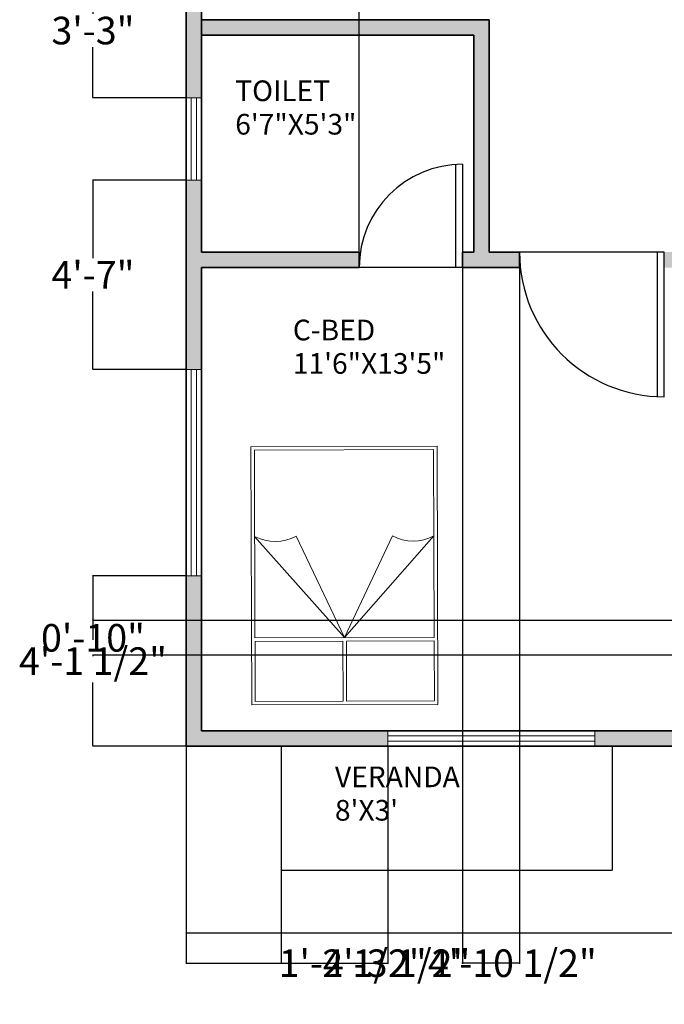
# Model space of a CAD drawing. Units: inches. Extents: x -27 to 662, y -19 to 539.
# Tile 1 of 4: x -27 to 160, y -19 to 267. Entities that reach past the tile are written whole.
import ezdxf

# ---------------------------------------------------------------- set-up
doc = ezdxf.new("R2010")
doc.units = ezdxf.units.IN
doc.header["$MEASUREMENT"] = 0
for name, color, linetype, lineweight in [('A-ANNO-DIMS', 2, 'Continuous', 18), ('A-AREA-IDEN', 230, 'Continuous', 18), ('A-DOOR', 6, 'Continuous', 25), ('A-FLOR', 4, 'Continuous', 25), ('A-FURN', 240, 'Continuous', 18), ('A-GLAZ', 240, 'Continuous', 18), ('A-WALL', 4, 'Continuous', 35)]:
    doc.layers.add(name, color=color, linetype=linetype, lineweight=lineweight)
doc.layers.add('A-WALL-PATT', color=2, linetype='Continuous', lineweight=13, true_color=0xf1eb1f)
doc.styles.get("Standard").update_dxf_attribs({"font": 'italic8.shx'})
doc.dimstyles.get("Standard").update_dxf_attribs({"dimtxt": 8, "dimasz": 0.18, "dimexe": 0.18, "dimexo": 0.0625, "dimgap": 0.09, "dimtad": 0, "dimtih": 1, "dimtoh": 1, "dimzin": 0, "dimdsep": 46, "dimlunit": 3, "dimtxsty": 'Standard', "dimcen": 0.09, "dimclrt": 4, "dimadec": 0, "dimazin": 0, "dimtfac": 1, "dimtofl": 0, "dimtmove": 0, "dimatfit": 3, "dimfxl": 1, "dimtolj": 1, "dimtzin": 0, "dimarcsym": 0})

# ---------------------------------------------------------------- blocks, each defined once
blk = doc.blocks.new('*D1')
at = {"layer": 'A-ANNO-DIMS', "color": 0, "lineweight": -2, "transparency": 16777216}
for p, q in [((21.29, 55.86), (21.29, 1.58)), ((417.29, 55.86), (417.29, 1.58)), ((21.47, 1.76), (209.67, 1.76)), ((417.11, 1.76), (228.9, 1.76))]:
    blk.add_line(p, q, dxfattribs=at)
at = {"layer": 'A-ANNO-DIMS', "color": 0, "transparency": 16777216}
for points in [[(21.47, 1.79), (21.47, 1.73), (21.29, 1.76)], [(417.11, 1.79), (417.11, 1.73), (417.29, 1.76)]]:
    blk.add_solid(points, dxfattribs=at)
at = {"layer": 'Defpoints', "color": 0, "transparency": 16777216}
for p in [(21.29, 55.92), (417.29, 55.92), (417.29, 1.76)]:
    blk.add_point(p, dxfattribs=at)
at = {"layer": 'A-ANNO-DIMS', "color": 0, "transparency": 16777216, "insert": (219.29, 1.76), "char_height": 8, "attachment_point": 5}
blk.add_mtext("\\A1;33'", dxfattribs=at)
blk = doc.blocks.new('BED-DOUBLE-54x75')
for p, q in [((26.5, 56.54), (26.5, 74)), ((27.5, 56.54), (27.5, 74)), ((1, 56.54), (26.5, 56.54)), ((1, 55.54), (53, 55.54)), ((27, 55.54), (1, 26.04)), ((13, 26.04), (27, 55.54)), ((27, 55.54), (53, 26.04)), ((41, 26.04), (27, 55.54)), ((27.5, 56.54), (53, 56.54))]:
    blk.add_line(p, q)
blk.add_lwpolyline([(0, 75), (54, 75), (54, 0), (0, 0)], close=True)
for points in [[(1, 56.54), (1, 74), (26.5, 74)], [(27.5, 74), (53, 74), (53, 56.54)], [(53, 55.54), (53, 1), (1, 1), (1, 55.54)]]:
    blk.add_lwpolyline(points)
for centre in [(7, 14.92), (47, 14.92)]:
    blk.add_arc(centre, 12.64, 61.656, 118.344)
blk = doc.blocks.new('DOOR-SWING-30IN')
for p, q in [((28, 29.93), (28, 0)), ((30, 30), (30, 0)), ((30, 0), (0, 0))]:
    blk.add_line(p, q)
blk.add_arc((30, 0), 30, 90, 180)
blk = doc.blocks.new('DOOR-SWING-42IN')
for p, q in [((0, 42), (0, 0)), ((2, 41.95), (2, 0)), ((0, 0), (42, 0))]:
    blk.add_line(p, q)
blk.add_arc((0, 0), 42, 0, 90)
blk = doc.blocks.new('WIN-60IN')
for p, q in [((0, 4.5), (0, 0)), ((60, 4.5), (0, 4.5)), ((0, 3), (60, 3)), ((60, 0), (60, 4.5)), ((0, 1.5), (60, 1.5)), ((0, 0), (60, 0))]:
    blk.add_line(p, q)
blk = doc.blocks.new('WIN-60IN-B')
for p, q in [((0, 0), (0, 60)), ((0, 60), (4.5, 60)), ((1.5, 0), (1.5, 60)), ((3, 0), (3, 60)), ((4.5, 60), (4.5, 0)), ((4.5, 0), (0, 0)), ((4.5, 0), (2.25, 0))]:
    blk.add_line(p, q)
blk = doc.blocks.new('WIN-24IN-B')
for p, q in [((0, 24), (4.5, 24)), ((0, 0), (0, 24)), ((0, 24), (2.25, 24)), ((1.5, 24), (1.5, 0)), ((3, 24), (3, 0)), ((4.5, 24), (4.5, 0)), ((4.5, 0), (0, 0))]:
    blk.add_line(p, q)
blk = doc.blocks.new('*D25')
at = {"layer": 'A-ANNO-DIMS', "color": 0, "lineweight": -2, "transparency": 16777216}
for p, q in [((21.29, 283.19), (21.29, 277.67)), ((25.79, 283.19), (25.79, 277.67)), ((21.47, 277.85), (25.61, 277.85)), ((25.79, 277.85), (25.97, 277.85))]:
    blk.add_line(p, q, dxfattribs=at)
at = {"layer": 'A-ANNO-DIMS', "color": 0, "transparency": 16777216}
for points in [[(21.47, 277.88), (21.47, 277.82), (21.29, 277.85)], [(25.61, 277.88), (25.61, 277.82), (25.79, 277.85)]]:
    blk.add_solid(points, dxfattribs=at)
at = {"layer": 'Defpoints', "color": 0, "transparency": 16777216}
for p in [(21.29, 283.25), (25.79, 283.25), (25.79, 277.85)]:
    blk.add_point(p, dxfattribs=at)
at = {"layer": 'A-ANNO-DIMS', "color": 4, "transparency": 16777216, "insert": (77.49, 277.85), "char_height": 8, "attachment_point": 5}
blk.add_mtext('\\A1;0\'-4 1/2" TYP.', dxfattribs=at)
blk = doc.blocks.new('*D36')
at = {"layer": 'A-ANNO-DIMS', "color": 0, "lineweight": -2, "transparency": 16777216}
for p, q in [((168.225254, 92.419463), (-5.892246, 92.419463)), ((-5.712246, 92.599463), (-5.712246, 92.779463)), ((168.225254, 82.419463), (-5.892246, 82.419463)), ((-5.712246, 82.239463), (-5.712246, 82.059463))]:
    blk.add_line(p, q, dxfattribs=at)
at = {"layer": 'A-ANNO-DIMS', "color": 0, "transparency": 16777216}
for points in [[(-5.742246, 92.599463), (-5.682246, 92.599463), (-5.712246, 92.419463)], [(-5.742246, 82.239463), (-5.682246, 82.239463), (-5.712246, 82.419463)]]:
    blk.add_solid(points, dxfattribs=at)
at = {"layer": 'Defpoints', "color": 0, "transparency": 16777216}
for p in [(-5.712246, 92.419463), (168.287754, 92.419463), (168.287754, 82.419463)]:
    blk.add_point(p, dxfattribs=at)
at = {"layer": 'A-ANNO-DIMS', "color": 4, "transparency": 16777216, "insert": (-5.712246, 87.419463), "char_height": 8, "attachment_point": 5}
blk.add_mtext('\\A1;0\'-10"', dxfattribs=at)
blk = doc.blocks.new('*D45')
at = {"layer": 'A-ANNO-DIMS', "color": 0, "lineweight": -2, "transparency": 16777216}
for p, q in [((21.23, 105.38), (-5.89, 105.38)), ((-5.71, 105.2), (-5.71, 86.84)), ((-5.71, 56.1), (-5.71, 74.47)), ((21.23, 55.92), (-5.89, 55.92))]:
    blk.add_line(p, q, dxfattribs=at)
at = {"layer": 'A-ANNO-DIMS', "color": 0, "transparency": 16777216}
for points in [[(-5.74, 105.2), (-5.68, 105.2), (-5.71, 105.38)], [(-5.74, 56.1), (-5.68, 56.1), (-5.71, 55.92)]]:
    blk.add_solid(points, dxfattribs=at)
at = {"layer": 'Defpoints', "color": 0, "transparency": 16777216}
for p in [(-5.71, 105.38), (21.29, 105.38), (21.29, 55.92)]:
    blk.add_point(p, dxfattribs=at)
at = {"layer": 'A-ANNO-DIMS', "color": 4, "transparency": 16777216, "insert": (-5.71, 80.65), "char_height": 8, "attachment_point": 5}
blk.add_mtext('\\A1;4\'-1 1/2"', dxfattribs=at)
blk = doc.blocks.new('*D46')
at = {"layer": 'A-ANNO-DIMS', "color": 0, "lineweight": -2, "transparency": 16777216}
for p, q in [((21.23, 220.27), (-5.89, 220.27)), ((-5.71, 220.09), (-5.71, 197.68)), ((-5.71, 165.56), (-5.71, 187.98)), ((21.23, 165.38), (-5.89, 165.38))]:
    blk.add_line(p, q, dxfattribs=at)
at = {"layer": 'A-ANNO-DIMS', "color": 0, "transparency": 16777216}
for points in [[(-5.74, 220.09), (-5.68, 220.09), (-5.71, 220.27)], [(-5.74, 165.56), (-5.68, 165.56), (-5.71, 165.38)]]:
    blk.add_solid(points, dxfattribs=at)
at = {"layer": 'Defpoints', "color": 0, "transparency": 16777216}
for p in [(-5.71, 220.27), (21.29, 220.27), (21.29, 165.38)]:
    blk.add_point(p, dxfattribs=at)
at = {"layer": 'A-ANNO-DIMS', "color": 4, "transparency": 16777216, "insert": (-5.71, 192.83), "char_height": 8, "attachment_point": 5}
blk.add_mtext('\\A1;4\'-7"', dxfattribs=at)
blk = doc.blocks.new('*D47')
at = {"layer": 'A-ANNO-DIMS', "color": 0, "lineweight": -2, "transparency": 16777216}
for p, q in [((21.23, 283.25), (-5.89, 283.25)), ((-5.71, 283.07), (-5.71, 268.61)), ((-5.71, 244.45), (-5.71, 258.91)), ((21.23, 244.27), (-5.89, 244.27))]:
    blk.add_line(p, q, dxfattribs=at)
at = {"layer": 'A-ANNO-DIMS', "color": 0, "transparency": 16777216}
for points in [[(-5.74, 283.07), (-5.68, 283.07), (-5.71, 283.25)], [(-5.74, 244.45), (-5.68, 244.45), (-5.71, 244.27)]]:
    blk.add_solid(points, dxfattribs=at)
at = {"layer": 'Defpoints', "color": 0, "transparency": 16777216}
for p in [(-5.71, 283.25), (21.29, 283.25), (21.29, 244.27)]:
    blk.add_point(p, dxfattribs=at)
at = {"layer": 'A-ANNO-DIMS', "color": 4, "transparency": 16777216, "insert": (-5.71, 263.76), "char_height": 8, "attachment_point": 5}
blk.add_mtext('\\A1;3\'-3"', dxfattribs=at)
blk = doc.blocks.new('*D48')
at = {"layer": 'A-ANNO-DIMS', "color": 0, "lineweight": -2, "transparency": 16777216}
for p, q in [((21.29, 55.86), (21.29, -7.26)), ((79.87, 55.86), (79.87, -7.26)), ((21.47, -7.08), (79.69, -7.08)), ((79.87, -7.08), (80.05, -7.08))]:
    blk.add_line(p, q, dxfattribs=at)
at = {"layer": 'A-ANNO-DIMS', "color": 0, "transparency": 16777216}
for points in [[(21.47, -7.05), (21.47, -7.11), (21.29, -7.08)], [(79.69, -7.05), (79.69, -7.11), (79.87, -7.08)]]:
    blk.add_solid(points, dxfattribs=at)
at = {"layer": 'Defpoints', "color": 0, "transparency": 16777216}
for p in [(21.29, 55.92), (79.87, 55.92), (79.87, -7.08)]:
    blk.add_point(p, dxfattribs=at)
at = {"layer": 'A-ANNO-DIMS', "color": 4, "transparency": 16777216, "insert": (115.95, -7.08), "char_height": 8, "attachment_point": 5}
blk.add_mtext('\\A1;4\'-10 1/2"', dxfattribs=at)
blk = doc.blocks.new('*D49')
at = {"layer": 'A-ANNO-DIMS', "color": 0, "lineweight": -2, "transparency": 16777216}
for p, q in [((21.29, 55.86), (21.29, -7.26)), ((48.89, 55.86), (48.89, -7.26)), ((21.47, -7.08), (48.71, -7.08)), ((48.89, -7.08), (49.07, -7.08))]:
    blk.add_line(p, q, dxfattribs=at)
at = {"layer": 'A-ANNO-DIMS', "color": 0, "transparency": 16777216}
for points in [[(21.47, -7.05), (21.47, -7.11), (21.29, -7.08)], [(48.71, -7.05), (48.71, -7.11), (48.89, -7.08)]]:
    blk.add_solid(points, dxfattribs=at)
at = {"layer": 'Defpoints', "color": 0, "transparency": 16777216}
for p in [(21.29, 55.92), (48.89, 55.92), (48.89, -7.08)]:
    blk.add_point(p, dxfattribs=at)
at = {"layer": 'A-ANNO-DIMS', "color": 4, "transparency": 16777216, "insert": (82.3, -7.08), "char_height": 8, "attachment_point": 5}
blk.add_mtext('\\A1;2\'-3 1/2"', dxfattribs=at)
blk = doc.blocks.new('*D56')
at = {"layer": 'A-ANNO-DIMS', "color": 0, "lineweight": -2, "transparency": 16777216}
for p, q in [((25.79, 199.48), (25.79, 527.1)), ((25.97, 526.92), (71.34, 526.92)), ((71.52, 199.48), (71.52, 527.1)), ((71.52, 526.92), (71.7, 526.92))]:
    blk.add_line(p, q, dxfattribs=at)
at = {"layer": 'A-ANNO-DIMS', "color": 0, "transparency": 16777216}
for points in [[(25.97, 526.95), (25.97, 526.89), (25.79, 526.92)], [(71.34, 526.95), (71.34, 526.89), (71.52, 526.92)]]:
    blk.add_solid(points, dxfattribs=at)
at = {"layer": 'Defpoints', "color": 0, "transparency": 16777216}
for p in [(71.52, 526.92), (25.79, 199.42), (71.52, 199.42)]:
    blk.add_point(p, dxfattribs=at)
at = {"layer": 'A-ANNO-DIMS', "color": 4, "transparency": 16777216, "insert": (104.93, 526.92), "char_height": 8, "attachment_point": 5}
blk.add_mtext('\\A1;3\'-9 1/2"', dxfattribs=at)
blk = doc.blocks.new('*D57')
at = {"layer": 'A-ANNO-DIMS', "color": 0, "lineweight": -2, "transparency": 16777216}
for p, q in [((101.52, 194.86), (101.52, -7.26)), ((118.05, 194.86), (118.05, -7.26)), ((101.52, -7.08), (101.34, -7.08)), ((117.87, -7.08), (101.7, -7.08))]:
    blk.add_line(p, q, dxfattribs=at)
at = {"layer": 'A-ANNO-DIMS', "color": 0, "transparency": 16777216}
for points in [[(101.7, -7.05), (101.7, -7.11), (101.52, -7.08)], [(117.87, -7.05), (117.87, -7.11), (118.05, -7.08)]]:
    blk.add_solid(points, dxfattribs=at)
at = {"layer": 'Defpoints', "color": 0, "transparency": 16777216}
for p in [(101.52, 194.92), (118.05, 194.92), (101.52, -7.08)]:
    blk.add_point(p, dxfattribs=at)
at = {"layer": 'A-ANNO-DIMS', "color": 4, "transparency": 16777216, "insert": (69.63, -7.08), "char_height": 8, "attachment_point": 5}
blk.add_mtext('\\A1;1\'-4 1/2"', dxfattribs=at)

msp = doc.modelspace()

# ---------------------------------------------------------------- hatches: boundary and pattern name
at = {"layer": 'A-WALL-PATT'}
h = msp.add_hatch(color=256, dxfattribs=at)
h.dxf.hatch_style = 1
h.paths.add_polyline_path([(79.868, 60.419), (25.788, 60.419), (25.788, 105.383), (21.288, 105.383), (21.288, 55.919), (79.868, 55.919)])
h.paths.add_polyline_path([(168.288, 194.919), (178.163, 194.919), (178.163, 199.419), (160.053, 199.419), (160.053, 194.919), (163.788, 194.919), (163.788, 60.419), (139.868, 60.419), (139.868, 58.169), (139.868, 55.919), (163.788, 55.919), (163.788, 19.919), (194.188, 19.919), (194.188, 24.419), (168.288, 24.419)])
h.paths.add_polyline_path([(298.321, 60.419), (274.788, 60.419), (274.788, 194.919), (278.414, 194.919), (278.414, 199.419), (270.288, 199.419), (259.929, 199.419), (259.929, 194.919), (270.288, 194.919), (270.288, 24.419), (242.188, 24.419), (242.188, 19.919), (274.788, 19.919), (274.788, 55.919), (298.321, 55.919)])
h.paths.add_polyline_path([(417.288, 94.965), (412.788, 94.965), (412.788, 60.419), (358.321, 60.419), (358.321, 55.919), (417.288, 55.919)])
h.paths.add_polyline_path([(417.288, 220.271), (412.788, 220.271), (412.788, 199.419), (365.562, 199.419), (365.562, 194.919), (412.788, 194.919), (412.788, 154.965), (417.288, 154.965)])
h.paths.add_polyline_path([(333.788, 262.419), (412.788, 262.419), (412.788, 244.271), (415.038, 244.271), (417.288, 244.271), (417.288, 283.252), (412.788, 283.252), (412.788, 266.919), (329.288, 266.919), (329.288, 262.419), (329.288, 199.419), (320.414, 199.419), (320.414, 194.919), (335.562, 194.919), (335.562, 199.419), (333.788, 199.419)])
h.paths.add_polyline_path([(333.788, 329.919), (412.788, 329.919), (412.788, 319.252), (415.038, 319.252), (417.288, 319.252), (417.288, 356.883), (415.038, 356.883), (412.788, 356.883), (412.788, 334.419), (320.72, 334.419), (320.72, 329.919), (329.288, 329.919), (329.288, 297.07), (333.788, 297.07)])
h.paths.add_polyline_path([(220.796, 406.919), (238.139, 406.919), (238.139, 411.419), (220.788, 411.419), (220.788, 495.419), (229.602, 495.419), (229.602, 499.919), (203.089, 499.919), (203.089, 495.419), (216.288, 495.419), (216.288, 411.419), (200.507, 411.419), (200.507, 406.919), (216.288, 406.919), (216.288, 199.419), (214.163, 199.419), (214.163, 194.919), (223.929, 194.919), (223.929, 199.419), (221.182, 199.419)])
h.paths.add_polyline_path([(109.288, 266.919), (104.788, 266.919), (25.788, 266.919), (25.788, 262.419), (104.788, 262.419), (104.788, 199.419), (101.522, 199.419), (101.522, 194.919), (118.053, 194.919), (118.053, 199.419), (109.288, 199.419)])
h.paths.add_polyline_path([(71.522, 199.419), (25.788, 199.419), (25.788, 220.271), (21.288, 220.271), (21.288, 165.383), (25.788, 165.383), (25.788, 194.919), (71.522, 194.919)])
h.paths.add_polyline_path([(25.788, 283.252), (21.288, 283.252), (21.288, 244.271), (23.538, 244.271), (25.788, 244.271)])
h.paths.add_polyline_path([(118.822, 334.419), (25.788, 334.419), (25.788, 495.419), (61.341, 495.419), (61.341, 499.919), (21.288, 499.919), (21.288, 319.252), (23.538, 319.252), (25.788, 319.252), (25.788, 329.919), (104.788, 329.919), (104.788, 296.919), (109.288, 296.919), (109.288, 329.919), (118.822, 329.919)])
h.paths.add_polyline_path([(168.288, 406.919), (170.507, 406.919), (170.507, 411.419), (168.288, 411.419), (168.288, 495.419), (179.089, 495.419), (179.089, 499.919), (121.341, 499.919), (121.341, 495.419), (163.788, 495.419), (163.788, 334.419), (160.822, 334.419), (160.822, 329.919), (168.288, 329.919)])
h.paths.add_polyline_path([(312.716, 499.919), (253.602, 499.919), (253.602, 495.419), (270.288, 495.419), (270.288, 411.419), (268.139, 411.419), (268.139, 406.919), (270.288, 406.919), (270.288, 329.919), (278.72, 329.919), (278.72, 334.419), (274.788, 334.419), (274.788, 495.419), (312.716, 495.419)])
h.paths.add_polyline_path([(417.288, 499.919), (372.716, 499.919), (372.716, 495.419), (412.788, 495.419), (412.788, 416.883), (417.288, 416.883)])

# ---------------------------------------------------------------- linework, layer by layer
at = {"layer": 'A-FLOR'}
for p, q in [((48.886, 55.919), (48.886, 19.919)), ((144.886, 55.919), (144.886, 19.919)), ((48.886, 19.919), (144.886, 19.919))]:
    msp.add_line(p, q, dxfattribs=at)
at = {"layer": 'A-WALL'}
for p, q in [((21.288, 499.919), (21.288, 55.919)), ((25.788, 329.919), (25.788, 199.419)), ((104.788, 266.919), (25.788, 266.919)), ((104.788, 266.919), (109.288, 266.919)), ((109.288, 266.919), (109.288, 199.419)), ((104.788, 262.419), (25.788, 262.419)), ((104.788, 262.419), (104.788, 199.419)), ((71.522, 199.419), (25.788, 199.419)), ((71.522, 199.419), (71.522, 194.919)), ((104.788, 199.419), (101.522, 199.419)), ((101.522, 199.419), (101.522, 194.919)), ((118.053, 199.419), (109.288, 199.419)), ((118.053, 199.419), (118.053, 194.919)), ((25.788, 194.919), (25.788, 60.419)), ((71.522, 194.919), (25.788, 194.919)), ((118.053, 194.919), (101.522, 194.919)), ((25.788, 60.419), (163.788, 60.419)), ((21.288, 55.919), (163.788, 55.919))]:
    msp.add_line(p, q, dxfattribs=at)

# ---------------------------------------------------------------- block references
at = {"layer": 'A-DOOR'}
msp.add_blockref('DOOR-SWING-30IN', (71.522, 194.919), dxfattribs=at)
at = {"layer": 'A-DOOR', "rotation": 180}
msp.add_blockref('DOOR-SWING-42IN', (160.053, 199.42), dxfattribs=at)
at = {"layer": 'A-FURN', "rotation": 180.1904805262934}
msp.add_blockref('BED-DOUBLE-54x75', (94.113, 143.097), dxfattribs=at)
at = {"layer": 'A-GLAZ'}
msp.add_blockref('WIN-24IN-B', (21.288, 220.271), dxfattribs=at)
for name, p, rotation in [('WIN-60IN', (21.287, 165.383), 269.9999999999998), ('WIN-60IN-B', (139.868, 55.92), 89.99999999999984)]:
    msp.add_blockref(name, p, dxfattribs=dict(at, rotation=rotation))

# ---------------------------------------------------------------- texts
at = {"layer": 'A-AREA-IDEN'}
for s, p in [('TOILET', (35.563, 243.274)), ('6\'7"X5\'3"', (35.563, 233.56)), ('C-BED', (52.28, 173.802)), ('11\'6"X13\'5"', (52.28, 164.088)), ('VERANDA', (64.492, 44.045)), ("8'X3'", (64.492, 34.33))]:
    msp.add_text(s, height=6, dxfattribs=at).set_placement(p)

# ---------------------------------------------------------------- dimensions: what is measured, and where the dimension line sits
at = {"layer": 'A-ANNO-DIMS'}
for base, p1, p2, override, picture, middle in [((71.522, 526.919), (25.788, 199.419), (71.522, 199.419), {"dimdec": 1, "dimlfac": 1, "dimrnd": 0, "dimzin": 1, "dimdsep": 46, "dimlunit": 4, "dimfrac": 2}, '*D56', (104.935, 526.919)), ((101.522, -7.081), (118.053, 194.919), (101.522, 194.919), {"dimdec": 1, "dimlfac": 1, "dimrnd": 0, "dimzin": 1, "dimdsep": 46, "dimlunit": 4, "dimfrac": 2}, '*D57', (69.633, -7.081)), ((417.288, 1.759), (21.288, 55.919), (417.288, 55.919), {"dimclrd": 0, "dimclre": 0, "dimclrt": 0}, '*D1', (219.288, 1.759)), ((79.868, -7.081), (21.288, 55.919), (79.868, 55.919), {"dimdec": 1, "dimlfac": 1, "dimrnd": 0, "dimzin": 1, "dimdsep": 46, "dimlunit": 4, "dimfrac": 2}, '*D48', (115.948, -7.081)), ((48.886, -7.081), (21.288, 55.919), (48.886, 55.919), {"dimdec": 1, "dimlfac": 1, "dimrnd": 0, "dimzin": 1, "dimdsep": 46, "dimlunit": 4, "dimfrac": 2}, '*D49', (82.299, -7.081))]:
    dim = msp.add_linear_dim(base=base, p1=p1, p2=p2, dimstyle='Standard', override=override, dxfattribs=at)
    dim.commit()
    dim.dimension.update_dxf_attribs({"geometry": picture, "text_midpoint": middle})
dim = msp.add_linear_dim(base=(25.788, 277.852), p1=(21.288, 283.252), p2=(25.788, 283.252), text='<> TYP.', dimstyle='Standard', override={"dimdec": 1, "dimlfac": 1, "dimrnd": 0, "dimzin": 1, "dimdsep": 46, "dimlunit": 4, "dimfrac": 2}, dxfattribs=at)
dim.commit()
dim.dimension.update_dxf_attribs({"geometry": '*D25', "text_midpoint": (77.486, 277.852)})
for base, p1, p2, picture, middle in [((-5.712, 283.252), (21.288, 244.271), (21.288, 283.252), '*D47', (-5.712, 263.762)), ((-5.712, 220.271), (21.288, 165.383), (21.288, 220.271), '*D46', (-5.712, 192.827)), ((-5.712, 105.383), (21.288, 55.919), (21.288, 105.383), '*D45', (-5.712, 80.651)), ((-5.712, 92.419), (168.288, 82.419), (168.288, 92.419), '*D36', (-5.712, 87.419))]:
    dim = msp.add_linear_dim(base=base, p1=p1, p2=p2, angle=90, dimstyle='Standard', override={"dimdec": 1, "dimlfac": 1, "dimrnd": 0, "dimzin": 1, "dimdsep": 46, "dimlunit": 4, "dimfrac": 2}, dxfattribs=at)
    dim.commit()
    dim.dimension.update_dxf_attribs({"geometry": picture, "text_midpoint": middle})

doc.saveas('drawing.dxf')
